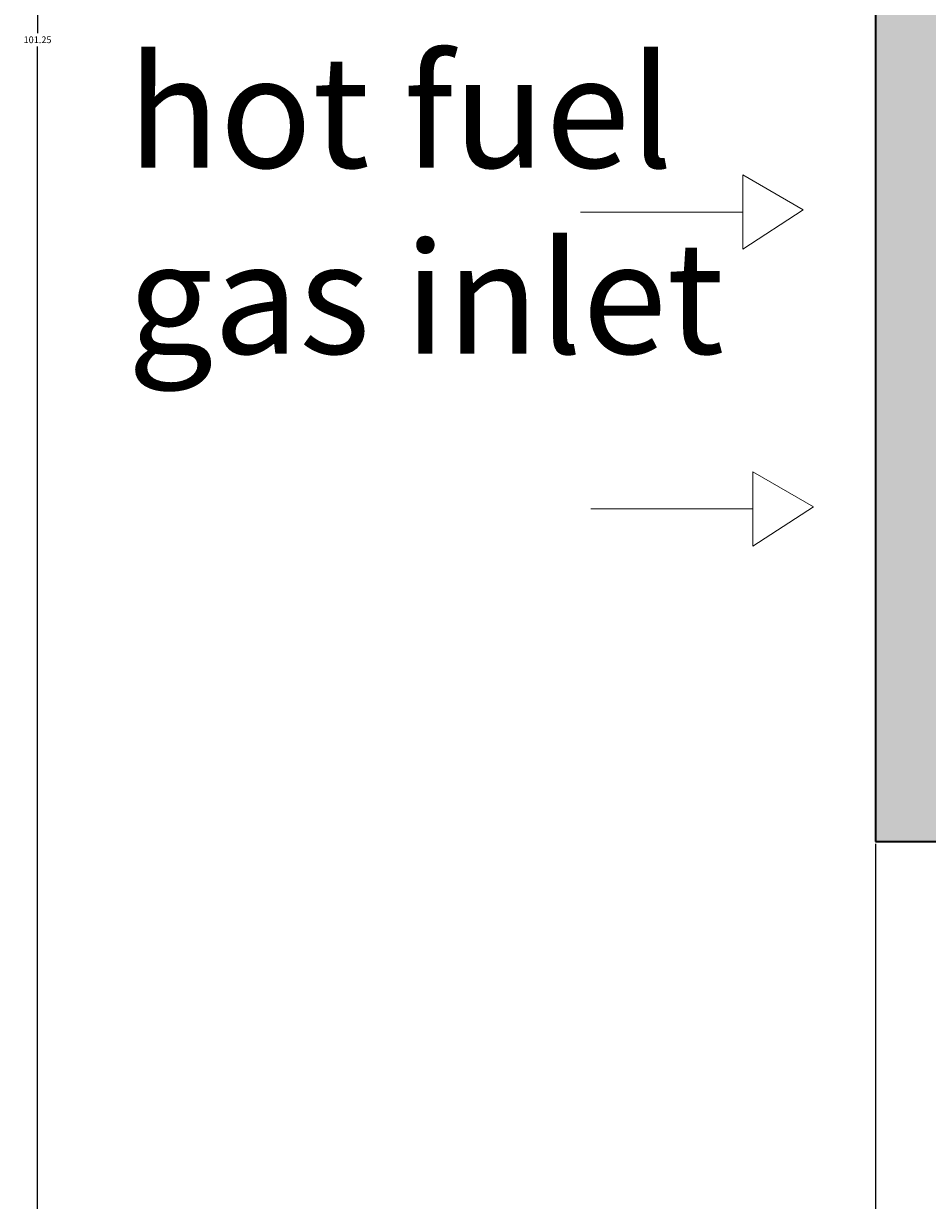
# Model space of a CAD drawing. Units: inches. Extents: x -1 to 292, y -3 to 199.
# Tile 5 of 52: x -1 to 23, y 45 to 77. Entities that reach past the tile are written whole.
import ezdxf

# ---------------------------------------------------------------- set-up
doc = ezdxf.new("R2010")
doc.units = ezdxf.units.IN
doc.header["$MEASUREMENT"] = 0
for name, color, linetype, lineweight in [('M-ANNO-SYMB', 1, 'Continuous', 18), ('M-ANNO-TEXT', 3, 'Continuous', 25), ('M-DIMS', 2, 'Continuous', 18), ('M-EQPM', 7, 'Continuous', 35), ('M-PATT', 8, 'Continuous', 13)]:
    doc.layers.add(name, color=color, linetype=linetype, lineweight=lineweight)
doc.styles.get("Standard").update_dxf_attribs({"font": 'arial.ttf'})
doc.dimstyles.get("Standard").update_dxf_attribs({"dimtxt": 0.18, "dimasz": 0.18, "dimexe": 0.18, "dimexo": 0.0625, "dimgap": 0.09, "dimtad": 0, "dimtih": 1, "dimtoh": 1, "dimdec": 4, "dimzin": 0, "dimdsep": 46, "dimtxsty": 'Standard', "dimcen": 0.09, "dimadec": 0, "dimazin": 0, "dimtfac": 1, "dimtdec": 4, "dimtofl": 0, "dimtmove": 0, "dimatfit": 3, "dimfxl": 1, "dimtolj": 1, "dimtzin": 0, "dimarcsym": 0})

# ---------------------------------------------------------------- blocks, each defined once
blk = doc.blocks.new('FLOW-ARROW-GAS')
for p, q in [((201.507, 38.14), (201.507, 36.14)), ((201.507, 38.14), (203.137, 37.199)), ((201.507, 37.14), (197.151, 37.14)), ((201.507, 36.14), (203.137, 37.199))]:
    blk.add_line(p, q)
blk = doc.blocks.new('DUCT-FLANGE')
for p, q in [((0, 34), (0, 0)), ((0, 34), (2.089, 34)), ((2.089, 34), (2.089, 0)), ((0, 0), (2.089, 0))]:
    blk.add_line(p, q)
blk = doc.blocks.new('*D7')
at = {"layer": 'Defpoints', "color": 0, "transparency": 16777216}
for p in [(21.861, 54.582), (205.115, 54.582), (21.861, 39.982)]:
    blk.add_point(p, dxfattribs=at)
at = {"layer": 'M-DIMS', "color": 0, "lineweight": -2, "transparency": 16777216}
for p, q in [((21.861, 54.52), (21.861, 39.802)), ((205.115, 54.52), (205.115, 39.802)), ((22.041, 39.982), (113.033, 39.982)), ((204.935, 39.982), (113.944, 39.982))]:
    blk.add_line(p, q, dxfattribs=at)
at = {"layer": 'M-DIMS', "color": 0, "transparency": 16777216}
for points in [[(22.041, 40.012), (22.041, 39.952), (21.861, 39.982)], [(204.935, 40.012), (204.935, 39.952), (205.115, 39.982)]]:
    blk.add_solid(points, dxfattribs=at)
at = {"layer": 'M-DIMS', "color": 0, "transparency": 16777216, "insert": (113.488, 39.982), "char_height": 0.18, "attachment_point": 5}
blk.add_mtext('\\A1;183.25', dxfattribs=at)
blk = doc.blocks.new('*D8')
at = {"layer": 'Defpoints', "color": 0, "transparency": 16777216}
for p in [(-0.662, 126.765), (111.488, 126.765), (69.013, 25.514)]:
    blk.add_point(p, dxfattribs=at)
at = {"layer": 'M-DIMS', "color": 0, "lineweight": -2, "transparency": 16777216}
for p, q in [((111.426, 126.765), (-0.842, 126.765)), ((-0.662, 126.585), (-0.662, 76.321)), ((-0.662, 25.694), (-0.662, 75.958)), ((68.951, 25.514), (-0.842, 25.514))]:
    blk.add_line(p, q, dxfattribs=at)
at = {"layer": 'M-DIMS', "color": 0, "transparency": 16777216}
for points in [[(-0.692, 126.585), (-0.632, 126.585), (-0.662, 126.765)], [(-0.692, 25.694), (-0.632, 25.694), (-0.662, 25.514)]]:
    blk.add_solid(points, dxfattribs=at)
at = {"layer": 'M-DIMS', "color": 0, "transparency": 16777216, "insert": (-0.662, 76.14), "char_height": 0.18, "attachment_point": 5}
blk.add_mtext('\\A1;101.25', dxfattribs=at)
blk = doc.blocks.new('*D14')
at = {"layer": 'Defpoints', "color": 0, "transparency": 16777216}
for p in [(21.861, 88.582), (21.861, 54.582), (36.461, 54.582)]:
    blk.add_point(p, dxfattribs=at)
at = {"layer": 'M-DIMS', "color": 0, "lineweight": -2, "transparency": 16777216}
for p, q in [((21.924, 88.582), (36.641, 88.582)), ((36.461, 88.402), (36.461, 71.764)), ((36.461, 54.762), (36.461, 71.4)), ((21.924, 54.582), (36.641, 54.582))]:
    blk.add_line(p, q, dxfattribs=at)
at = {"layer": 'M-DIMS', "color": 0, "transparency": 16777216}
for points in [[(36.431, 88.402), (36.491, 88.402), (36.461, 88.582)], [(36.431, 54.762), (36.491, 54.762), (36.461, 54.582)]]:
    blk.add_solid(points, dxfattribs=at)
at = {"layer": 'M-DIMS', "color": 0, "transparency": 16777216, "insert": (36.461, 71.582), "char_height": 0.18, "attachment_point": 5}
blk.add_mtext('\\A1;34', dxfattribs=at)
blk = doc.blocks.new('*D23')
at = {"layer": 'Defpoints', "color": 0, "transparency": 16777216}
for p in [(21.861, 54.582), (64.679, 51.267), (64.679, -2.71)]:
    blk.add_point(p, dxfattribs=at)
at = {"layer": 'M-DIMS', "color": 0, "lineweight": -2, "transparency": 16777216}
for p, q in [((21.861, 54.52), (21.861, -2.89)), ((64.679, 51.205), (64.679, -2.89)), ((22.041, -2.71), (42.874, -2.71)), ((64.499, -2.71), (43.666, -2.71))]:
    blk.add_line(p, q, dxfattribs=at)
at = {"layer": 'M-DIMS', "color": 0, "transparency": 16777216}
for points in [[(22.041, -2.68), (22.041, -2.74), (21.861, -2.71)], [(64.499, -2.68), (64.499, -2.74), (64.679, -2.71)]]:
    blk.add_solid(points, dxfattribs=at)
at = {"layer": 'M-DIMS', "color": 0, "transparency": 16777216, "insert": (43.27, -2.71), "char_height": 0.18, "attachment_point": 5}
blk.add_mtext('\\A1;42.82', dxfattribs=at)

msp = doc.modelspace()

# ---------------------------------------------------------------- hatches: boundary and pattern name
at = {"layer": 'M-PATT'}
h = msp.add_hatch(color=256, dxfattribs=at)
h.set_gradient(color1=(76, 38, 47), color2=(76, 38, 47), tint=1, name='CYLINDER')
h.paths.add_polyline_path([(40.8628, 91.6478), (40.3591, 92.5203), (23.9502, 85.5552), (23.9502, 84.4688)])
h.paths.add_polyline_path([(52.8586, 93.6403), (42.9977, 93.6403), (40.3591, 92.5203), (40.8628, 91.6478), (43.2011, 92.6403), (54.4604, 92.6403, -0.0601508)])
h.paths.add_polyline_path([(23.9502, 88.5821), (21.8612, 88.5821), (21.8612, 54.5821), (23.9502, 54.5821)])
h.paths.add_polyline_path([(23.9502, 58.376), (23.9502, 57.2213), (42.9332, 46.2615), (50.4659, 46.2615, -0.0351813), (50.9409, 47.2615), (43.2011, 47.2615)])
h.paths.add_polyline_path([(179.5897, 93.6403), (174.1181, 93.6403, -0.0601508), (172.5163, 92.6403), (179.5897, 92.6403)])
h.paths.add_polyline_path([(183.979, 93.6403), (181.5897, 93.6403), (181.5897, 92.6403), (183.7755, 92.6403), (203.0265, 84.4688), (203.0265, 85.5552)])
h.paths.add_polyline_path([(205.1155, 88.5821), (203.0265, 88.5821), (203.0265, 54.5821), (205.1155, 54.5821)])
h.paths.add_polyline_path([(203.0265, 57.2213), (203.0265, 58.376), (183.7755, 47.2615), (181.5897, 47.2615), (181.5897, 46.2615), (184.0435, 46.2615)])
h.paths.add_polyline_path([(179.5897, 47.2615), (176.0358, 47.2615, -0.0351813), (176.5107, 46.2615), (179.5897, 46.2615)])

# ---------------------------------------------------------------- block references
at = {"layer": 'M-ANNO-SYMB'}
for p in [(-183.2135, 34.3679), (-182.9398, 26.3883)]:
    msp.add_blockref('FLOW-ARROW-GAS', p, dxfattribs=at)
at = {"layer": 'M-EQPM'}
msp.add_blockref('DUCT-FLANGE', (21.861, 54.582), dxfattribs=at)

# ---------------------------------------------------------------- texts
at = {"layer": 'M-ANNO-TEXT', "insert": (1.7537, 75.7005), "char_height": 3, "attachment_point": 1}
msp.add_mtext_dynamic_manual_height_columns('hot fuel\\Pgas inlet', width=47.899539, gutter_width=1, heights=[0], dxfattribs=at)

# ---------------------------------------------------------------- dimensions: what is measured, and where the dimension line sits
at = {"layer": 'M-DIMS'}
for base, p1, p2, angle, override, picture, middle in [((-0.6625, 126.765), (69.013, 25.5141), (111.4883, 126.765), 90, {"dimdec": 2, "dimlfac": 1, "dimrnd": 0, "dimzin": 0, "dimdsep": 46, "dimlunit": 2}, '*D8', (-0.6625, 76.1396)), ((36.4612, 54.5821), (21.8612, 88.5821), (21.8612, 54.5821), 270, {"dimdec": 0, "dimlfac": 1, "dimrnd": 0, "dimzin": 0, "dimdsep": 46, "dimlunit": 2}, '*D14', (36.4612, 71.5821)), ((21.8612, 39.9821), (205.1155, 54.5821), (21.8612, 54.5821), 180, {"dimdec": 2, "dimlfac": 1, "dimrnd": 0, "dimzin": 0, "dimdsep": 46, "dimlunit": 2}, '*D7', (113.4883, 39.9821))]:
    dim = msp.add_linear_dim(base=base, p1=p1, p2=p2, angle=angle, dimstyle='Standard', override=override, dxfattribs=at)
    dim.commit()
    dim.dimension.update_dxf_attribs({"geometry": picture, "text_midpoint": middle})
dim = msp.add_linear_dim(base=(64.6788, -2.7104), p1=(21.8612, 54.5821), p2=(64.6788, 51.2672), dimstyle='Standard', override={"dimdec": 2, "dimlfac": 1, "dimrnd": 0, "dimzin": 0, "dimdsep": 46, "dimlunit": 2}, dxfattribs=at)
dim.commit()
dim.dimension.update_dxf_attribs({"geometry": '*D23', "text_midpoint": (43.27, -2.7104)})

doc.saveas('drawing.dxf')
